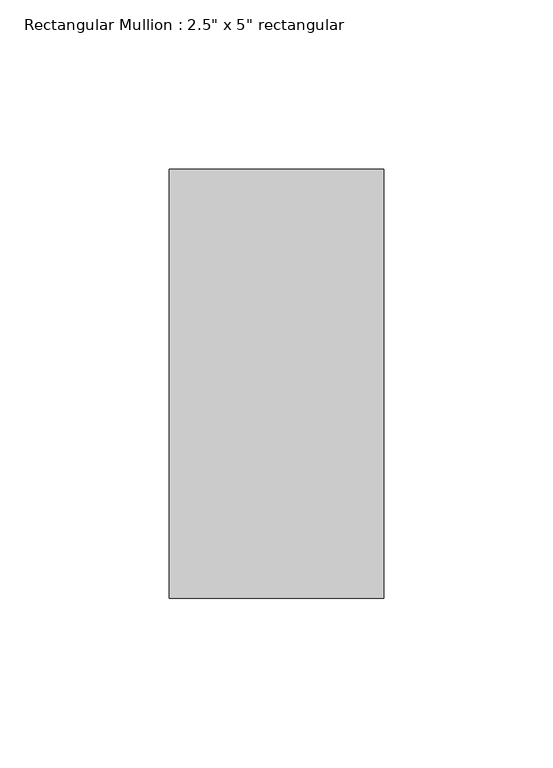
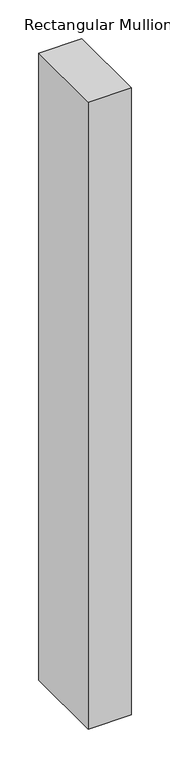
"""IFC4 building model written with IfcOpenShell, lengths in millimetres: member geometry."""

from ifc_helpers import new_model, si_unit, frame, origin, place, context, project, spatial, polyline, outline, extrude, source, transform, mapped, element, save


def member_413afe15(model_context):
    return source(origin(), model_context, "Body", "SweptSolid", [
        extrude(outline(polyline([(0.0, 63.5), (0.0, -63.5), (-63.5, -63.5), (-63.5, 63.5), (0.0, 63.5)])), frame((0.0, 0.0, -984.4396511), z_axis=(0.0, 0.0, 1.0), x_axis=(1.0, 0.0, 0.0)), (0.0, 0.0, 1.0), 984.4396511),
    ])


if __name__ == "__main__":
    model = new_model("IFC4")
    model_context = context("Model", 3, world=origin())
    ifc_project = project(units=[si_unit("LENGTHUNIT", "METRE", prefix="MILLI")], contexts=[model_context])
    site = spatial("IfcSite", under=ifc_project)
    building = spatial("IfcBuilding", under=site)
    placement = place(None, origin())
    member_shape = member_413afe15(model_context)
    element("IfcMember", 1, ObjectType="Rectangular Mullion : 2.5\" x 5\" rectangular", at=placement, inside=building, context=model_context, shape_type="MappedRepresentation", body=[
        mapped(member_shape, transform((0.0, 0.0, 0.0), x_axis=(1.0, 0.0, 0.0), y_axis=(0.0, 1.0, 0.0), z_axis=(0.0, 0.0, 1.0))),
    ])
    save(model, "model.ifc")

# Revit data of these elements
# Type "Rectangular Mullion : 2.5\" x 5\" rectangular"
#   built-in parameter 1007304 = 0.416667 (stored number, unit not read)
#   built-in parameter 1007301 = 0.104167 (stored number, unit not read)
#   built-in parameter 1007300 = 0.104167 (stored number, unit not read)
# Element 1 (IfcMember, "Rectangular Mullion : 2.5\" x 5\" rectangular")
#   Materials on its faces: "Aluminum"
# Materials
#   "Aluminum": class "Metal", colour RGB 247 247 247, transparency 0, Description = "Aluminum 6061", Cost = 0
